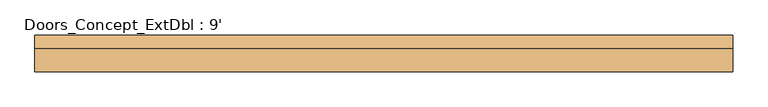
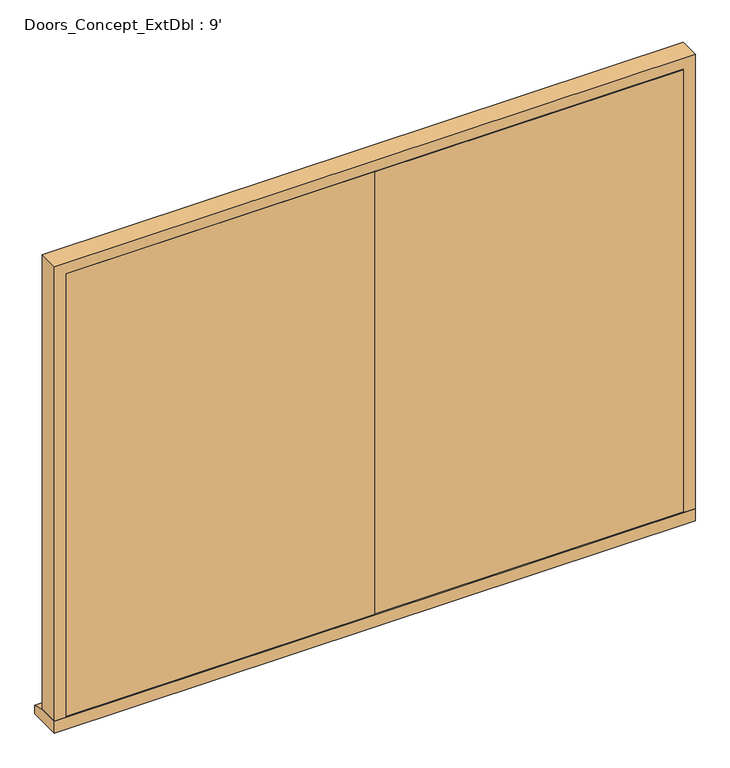
"""IFC4 building model written with IfcOpenShell, lengths in millimetres: door geometry, Doors_Concept_ExtDbl : 9'."""

from ifc_helpers import new_model, si_unit, frame, origin, place, context, project, spatial, polyline, outline, extrude, faceted_brep, source, transform, mapped, element, save


def doors_concept_extdbl_9_dbcc4ac8(model_context):
    return source(origin(), model_context, "Body", "SolidModel", [
        faceted_brep([(1301.1, 81.68, 54.5), (1371.6, 81.68, 54.5), (1371.6, -7.32, 54.5), (1323.1, -7.32, 54.5), (1323.1, 39.68, 54.5), (1301.1, 39.68, 54.5), (1301.1, 81.68, 2039.5), (-1301.1, 81.68, 2039.5), (-1301.1, 81.68, 54.5), (-1371.6, 81.68, 54.5), (-1371.6, 81.68, 2110.0), (1371.6, 81.68, 2110.0), (1371.6, -7.32, 2110.0), (-1371.6, -7.32, 2110.0), (-1371.6, -7.32, 54.5), (-1323.1, -7.32, 54.5), (-1323.1, -7.32, 2061.5), (1323.1, -7.32, 2061.5), (1323.1, 39.68, 2061.5), (-1323.1, 39.68, 2061.5), (-1323.1, 39.68, 54.5), (-1301.1, 39.68, 54.5), (-1301.1, 39.68, 2039.5), (1301.1, 39.68, 2039.5)], [[[0, 1, 2, 3, 4, 5]], [[1, 0, 6, 7, 8, 9, 10, 11]], [[2, 1, 11, 12]], [[3, 2, 12, 13, 14, 15, 16, 17]], [[4, 3, 17, 18]], [[5, 4, 18, 19, 20, 21, 22, 23]], [[0, 5, 23, 6]], [[7, 22, 21, 8]], [[8, 21, 20, 15, 14, 9]], [[13, 10, 9, 14]], [[19, 16, 15, 20]], [[12, 11, 10, 13]], [[18, 17, 16, 19]], [[6, 23, 22, 7]]]),
        extrude(outline(polyline([(1320.1, -7.32), (1.5, -7.32), (1.5, 36.68), (1320.1, 36.68), (1320.1, -7.32)])), frame((0.0, 0.0, 58.5), z_axis=(0.0, 0.0, 1.0), x_axis=(1.0, 0.0, 0.0)), (0.0, 0.0, 1.0), 2000.0),
        extrude(outline(polyline([(-1.5, -7.32), (-1320.1, -7.32), (-1320.1, 36.68), (-1.5, 36.68), (-1.5, -7.32)])), frame((0.0, 0.0, 58.5), z_axis=(0.0, 0.0, 1.0), x_axis=(1.0, 0.0, 0.0)), (0.0, 0.0, 1.0), 2000.0),
        extrude(outline(polyline([(-7.32, 0.0), (-7.32, 54.5), (81.68, 54.5), (136.68, 38.5947221), (136.68, 0.0), (-7.32, 0.0)])), frame((-1371.6, 0.0, 0.0), z_axis=(1.0, 0.0, 0.0), x_axis=(0.0, 1.0, 0.0)), (0.0, 0.0, 1.0), 2743.2),
    ])


if __name__ == "__main__":
    model = new_model("IFC4")
    model_context = context("Model", 3, world=origin())
    ifc_project = project(units=[si_unit("LENGTHUNIT", "METRE", prefix="MILLI")], contexts=[model_context])
    site = spatial("IfcSite", under=ifc_project)
    building = spatial("IfcBuilding", under=site)
    placement = place(None, origin())
    doors_concept_extdbl_9_shape = doors_concept_extdbl_9_dbcc4ac8(model_context)
    element("IfcDoor", 1, ObjectType="Doors_Concept_ExtDbl : 9'", at=placement, inside=building, context=model_context, shape_type="MappedRepresentation", body=[
        mapped(doors_concept_extdbl_9_shape, transform((0.0, 0.0, 0.0), x_axis=(1.0, 0.0, 0.0), y_axis=(0.0, 1.0, 0.0), z_axis=(0.0, 0.0, 1.0))),
    ])
    save(model, "model.ifc")

# Revit data of these elements
# Type "Doors_Concept_ExtDbl : 9'"
#   Type Mark = "54"
#   Type Comments = "External Double"
#   Operation = "DoubleDoorSingleSwing"
#   Construction Type Id = "GSP4R"
#   Keynote = "L10"
#   Analytic Construction = "1/8 in Pilkington single glazing"
#   Visual Light Transmittance = 0.9
#   Thickness = 0.144357 ft
#   Solar Heat Gain Coefficient = 0.78
#   Rough Width = 9.0 ft
#   Rough Height = 6.922572 ft
#   Heat Transfer Coefficient (U) = 3.6886 W/(m²·K)
#   FrameWidth = 0.137795 ft
#   FrameOffset - External = 0.082021 ft
#   Height = 6.922572 ft
#   Width = 9.0 ft
#   Define Thermal Properties by = 1
#   Function = 1
#   Material Door = Door - Glazing
#   Material Frame = Concept
#   Wall Closure = (empty or 0)
# Element 1 (IfcDoor, "Doors_Concept_ExtDbl : 9'")
#   Materials on its faces: "Concept", "Door - Glazing"
# Materials
#   "Door - Glazing": colour RGB 0 0 255, transparency 0.75
#   "Concept": colour RGB 128 128 255, transparency 0.5
